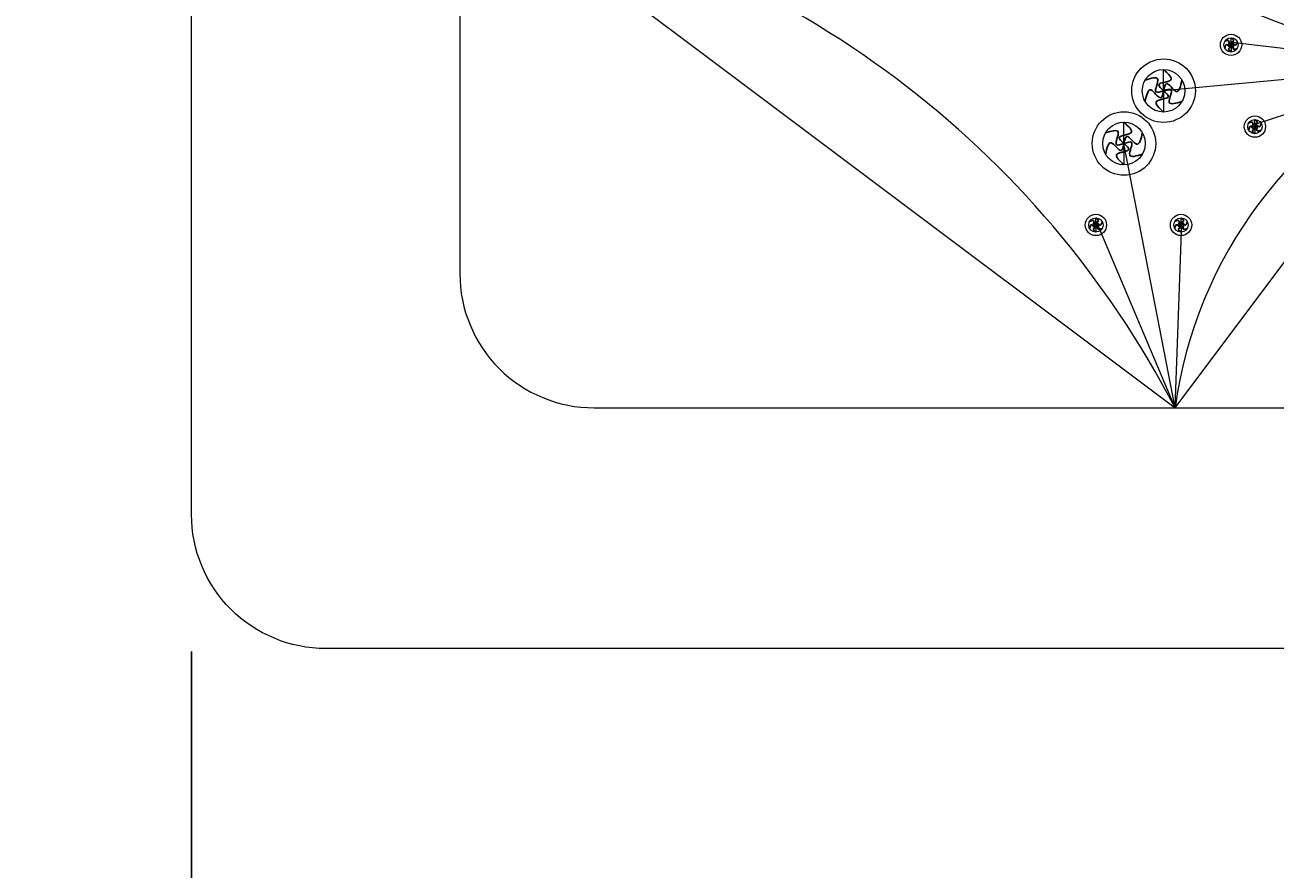
# Model space of a CAD drawing. Units: inches. Extents: x -61 to 1599, y -1316 to 257.
# Tile 99 of 204: x 142 to 170, y -166 to -147. Entities that reach past the tile are written whole.
import ezdxf

# ---------------------------------------------------------------- set-up
doc = ezdxf.new("R2010")
doc.units = ezdxf.units.IN
doc.header["$MEASUREMENT"] = 0
doc.layers.add('A-ANNO-DIMS', color=2, linetype='Continuous', lineweight=18)
doc.layers.add('FURNITURE', color=83, linetype='Continuous', lineweight=18)
doc.layers.add('FUR', color=83, linetype='Continuous')
doc.styles.get("Standard").update_dxf_attribs({"font": 'arial.ttf'})
doc.dimstyles.get("Standard").update_dxf_attribs({"dimtxt": 0.18, "dimasz": 0.18, "dimexe": 0.18, "dimexo": 0.0625, "dimgap": 0.09, "dimtad": 0, "dimtih": 1, "dimtoh": 1, "dimdec": 0, "dimzin": 0, "dimdsep": 46, "dimlunit": 3, "dimtxsty": 'Standard', "dimcen": 0.09, "dimadec": 0, "dimazin": 0, "dimtfac": 1, "dimtdec": 0, "dimtofl": 0, "dimtmove": 0, "dimatfit": 3, "dimfxl": 1, "dimtolj": 1, "dimtzin": 0, "dimarcsym": 0})

# ---------------------------------------------------------------- blocks, each defined once
blk = doc.blocks.new('*U124')
at = {"layer": 'FUR'}
blk.add_open_spline([(0.005, 0.08), (-0.03, 0.048), (-0.098, -0.015), (0.075, -0.018), (0.024, -0.063), (0.005, -0.08)], degree=3, knots=[0, 0, 0, 0, 0.0954578, 0.1898773, 0.2470677, 0.2470677, 0.2470677, 0.2470677], dxfattribs=at)
blk = doc.blocks.new('*U125')
at = {"layer": 'FUR', "transparency": 16777216}
for p, rotation in [((222.173, -79.977), 60), ((222.312, -79.968), 300), ((222.178, -80.056), 120), ((222.25, -80.092), 180), ((222.317, -80.048), 240)]:
    blk.add_blockref('*U124', p, dxfattribs=dict(at, rotation=rotation))
blk.add_blockref('*U124', (222.24, -79.932), dxfattribs=at)
blk = doc.blocks.new('*U134')
at = {"layer": 'FUR'}
blk.add_open_spline([(0.015, 0.238), (-0.088, 0.143), (-0.292, -0.045), (0.224, -0.053), (0.072, -0.187), (0.015, -0.238)], degree=3, knots=[0, 0, 0, 0, 0.2846533, 0.5662105, 0.736751, 0.736751, 0.736751, 0.736751], dxfattribs=at)
blk = doc.blocks.new('*U123')
at = {"layer": 'FUR', "transparency": 16777216}
blk.add_blockref('*U134', (662.716, -238.357), dxfattribs=at)
for p, rotation in [((662.517, -238.489), 60), ((662.929, -238.463), 300), ((662.531, -238.727), 120), ((662.745, -238.833), 180), ((662.944, -238.702), 240)]:
    blk.add_blockref('*U134', p, dxfattribs=dict(at, rotation=rotation))
blk = doc.blocks.new('*U130')
at = {"layer": 'FUR'}
blk.add_open_spline([(0.015, 0.238), (-0.088, 0.143), (-0.292, -0.045), (0.224, -0.053), (0.072, -0.187), (0.015, -0.238)], degree=3, knots=[0, 0, 0, 0, 0.2846533, 0.5662105, 0.736751, 0.736751, 0.736751, 0.736751], dxfattribs=at)
blk = doc.blocks.new('*U131')
at = {"layer": 'FUR', "transparency": 16777216}
blk.add_blockref('*U130', (662.716, -238.357), dxfattribs=at)
for p, rotation in [((662.517, -238.489), 60), ((662.929, -238.463), 300), ((662.531, -238.727), 120), ((662.745, -238.833), 180), ((662.944, -238.702), 240)]:
    blk.add_blockref('*U130', p, dxfattribs=dict(at, rotation=rotation))
blk = doc.blocks.new('*U126')
at = {"layer": 'FUR'}
blk.add_open_spline([(0.005, 0.08), (-0.03, 0.048), (-0.098, -0.015), (0.075, -0.018), (0.024, -0.063), (0.005, -0.08)], degree=3, knots=[0, 0, 0, 0, 0.0954578, 0.1898773, 0.2470677, 0.2470677, 0.2470677, 0.2470677], dxfattribs=at)
blk = doc.blocks.new('*U127')
at = {"layer": 'FUR', "transparency": 16777216}
for p, rotation in [((222.173, -79.977), 60), ((222.312, -79.968), 300), ((222.178, -80.056), 120), ((222.25, -80.092), 180), ((222.317, -80.048), 240)]:
    blk.add_blockref('*U126', p, dxfattribs=dict(at, rotation=rotation))
blk.add_blockref('*U126', (222.24, -79.932), dxfattribs=at)
blk = doc.blocks.new('*U146')
at = {"layer": 'FUR'}
blk.add_open_spline([(0.005, 0.08), (-0.03, 0.048), (-0.098, -0.015), (0.075, -0.018), (0.024, -0.063), (0.005, -0.08)], degree=3, knots=[0, 0, 0, 0, 0.0954578, 0.1898773, 0.2470677, 0.2470677, 0.2470677, 0.2470677], dxfattribs=at)
blk = doc.blocks.new('*U147')
at = {"layer": 'FUR', "transparency": 16777216}
for p, rotation in [((222.173, -79.977), 60), ((222.312, -79.968), 300), ((222.178, -80.056), 120), ((222.25, -80.092), 180), ((222.317, -80.048), 240)]:
    blk.add_blockref('*U146', p, dxfattribs=dict(at, rotation=rotation))
blk.add_blockref('*U146', (222.24, -79.932), dxfattribs=at)
blk = doc.blocks.new('*U144')
at = {"layer": 'FUR'}
blk.add_open_spline([(0.005, 0.08), (-0.03, 0.048), (-0.098, -0.015), (0.075, -0.018), (0.024, -0.063), (0.005, -0.08)], degree=3, knots=[0, 0, 0, 0, 0.0954578, 0.1898773, 0.2470677, 0.2470677, 0.2470677, 0.2470677], dxfattribs=at)
blk = doc.blocks.new('*U145')
at = {"layer": 'FUR', "transparency": 16777216}
for p, rotation in [((222.173, -79.977), 60), ((222.312, -79.968), 300), ((222.178, -80.056), 120), ((222.25, -80.092), 180), ((222.317, -80.048), 240)]:
    blk.add_blockref('*U144', p, dxfattribs=dict(at, rotation=rotation))
blk.add_blockref('*U144', (222.24, -79.932), dxfattribs=at)
blk = doc.blocks.new('SOFA-THREE-SEAT')
for p, q in [((23.243, 13.498), (23.243, 13.658)), ((23.243, 13.498), (23.243, 13.338)), ((27.729, 13.028), (23.263, 13.551)), ((27.729, 13.028), (21.735, 12.472)), ((21.735, 12.472), (21.735, 12.949)), ((27.729, 13.028), (23.795, 11.722)), ((21.735, 12.472), (21.735, 11.996)), ((20.849, 11.292), (20.849, 11.769)), ((23.776, 11.67), (23.776, 11.83)), ((23.776, 11.67), (23.776, 11.51)), ((21.991, 5.382), (20.849, 11.292)), ((20.849, 11.292), (20.849, 10.816)), ((20.221, 9.471), (20.221, 9.631)), ((21.991, 5.382), (20.241, 9.523)), ((21.991, 5.382), (22.145, 9.523)), ((22.125, 9.471), (22.125, 9.631)), ((20.221, 9.471), (20.221, 9.311)), ((22.125, 9.471), (22.125, 9.311))]:
    blk.add_line(p, q)
blk.add_lwpolyline([(78, 8.382), (78, 23, -0.414214), (81, 26), (81, 26, -0.414214), (84, 23), (84, 3, -0.414214), (81, 0), (3, 0, -0.414214), (0, 3), (0, 23, -0.414214), (3, 26), (3, 26, -0.414214), (6, 23), (6, 8.382, 0.414214), (9, 5.382), (75, 5.382, 0.414214)], format="xyb", close=True)
blk.add_lwpolyline([(27.729, 13.028), (12.664, 24.333), (6.926, 16.687), (21.991, 5.382)], close=True)
for centre, radius in [((23.243, 13.498), 0.238), ((23.243, 13.498), 0.16), ((21.735, 12.472), 0.71), ((21.735, 12.472), 0.476), ((20.849, 11.292), 0.71), ((20.849, 11.292), 0.476), ((23.776, 11.67), 0.238), ((23.776, 11.67), 0.16), ((20.221, 9.471), 0.238), ((20.221, 9.471), 0.16), ((22.125, 9.471), 0.238), ((22.125, 9.471), 0.16)]:
    blk.add_circle(centre, radius)
for centre, radius, start, end in [((31.951, 34.345), 21.731, 207.4316, 258.7956), ((2.703, -4.63), 21.731, 27.4316, 78.7956), ((31.717, 4.059), 9.816, 113.9742, 172.253)]:
    blk.add_arc(centre, radius, start, end)
at = {"xscale": -1, "rotation": 180}
for name, p in [('*U147', (-199.001, -66.514)), ('*U131', (-640.996, -226.123)), ('*U123', (-641.881, -227.303)), ('*U145', (-198.469, -68.342)), ('*U125', (-202.024, -70.541)), ('*U127', (-200.12, -70.541))]:
    blk.add_blockref(name, p, dxfattribs=at)
blk = doc.blocks.new('*D670')
at = {"layer": 'A-ANNO-DIMS', "color": 0, "lineweight": -2, "transparency": 16777216}
for p, q in [((145.375, -161.442), (145.375, -174.159)), ((229.375, -161.442), (229.375, -174.159)), ((145.555, -173.979), (186.47, -173.979)), ((229.195, -173.979), (188.279, -173.979))]:
    blk.add_line(p, q, dxfattribs=at)
at = {"layer": 'A-ANNO-DIMS', "color": 0, "transparency": 16777216}
for points in [[(145.555, -173.949), (145.555, -174.009), (145.375, -173.979)], [(229.195, -173.949), (229.195, -174.009), (229.375, -173.979)]]:
    blk.add_solid(points, dxfattribs=at)
at = {"layer": 'DEFPOINTS', "color": 0, "transparency": 16777216}
for p in [(145.375, -161.379), (229.375, -161.379), (229.375, -173.979)]:
    blk.add_point(p, dxfattribs=at)
at = {"layer": 'A-ANNO-DIMS', "color": 0, "transparency": 16777216, "insert": (187.375, -173.979), "char_height": 0.18, "attachment_point": 5}
blk.add_mtext('\\A1;SOFA 84 TYP.', dxfattribs=at)
blk = doc.blocks.new('*D687')
at = {"layer": 'A-ANNO-DIMS', "color": 0, "lineweight": -2, "transparency": 16777216}
for p, q in [((289.418, 181.677), (-61.077, 181.677)), ((-60.897, 181.497), (-60.897, -528.952)), ((-60.897, -1239.765), (-60.897, -529.316)), ((319.64, -1239.945), (-61.077, -1239.945))]:
    blk.add_line(p, q, dxfattribs=at)
at = {"layer": 'A-ANNO-DIMS', "color": 0, "transparency": 16777216}
for points in [[(-60.927, 181.497), (-60.867, 181.497), (-60.897, 181.677)], [(-60.927, -1239.765), (-60.867, -1239.765), (-60.897, -1239.945)]]:
    blk.add_solid(points, dxfattribs=at)
at = {"layer": 'DEFPOINTS', "color": 0, "transparency": 16777216}
for p in [(289.481, 181.677), (-60.897, -1239.945), (319.703, -1239.945)]:
    blk.add_point(p, dxfattribs=at)
at = {"layer": 'A-ANNO-DIMS', "color": 0, "transparency": 16777216, "insert": (-60.897, -529.134), "char_height": 0.18, "attachment_point": 5}
blk.add_mtext('\\A1;1421.6', dxfattribs=at)
blk = doc.blocks.new('*D700')
at = {"layer": 'A-ANNO-DIMS', "color": 0, "lineweight": -2, "transparency": 16777216}
for p, q in [((14.703, -616.882), (14.703, 257.457)), ((179.752, -616.882), (179.752, 257.457)), ((14.883, 257.277), (96.772, 257.277)), ((179.572, 257.277), (97.683, 257.277))]:
    blk.add_line(p, q, dxfattribs=at)
at = {"layer": 'A-ANNO-DIMS', "color": 0, "transparency": 16777216}
for points in [[(14.883, 257.307), (14.883, 257.247), (14.703, 257.277)], [(179.572, 257.307), (179.572, 257.247), (179.752, 257.277)]]:
    blk.add_solid(points, dxfattribs=at)
at = {"layer": 'DEFPOINTS', "color": 0, "transparency": 16777216}
for p in [(179.752, 257.277), (14.703, -616.945), (179.752, -616.945)]:
    blk.add_point(p, dxfattribs=at)
at = {"layer": 'A-ANNO-DIMS', "color": 0, "transparency": 16777216, "insert": (97.227, 257.277), "char_height": 0.18, "attachment_point": 5}
blk.add_mtext('\\A1;165.05', dxfattribs=at)

msp = doc.modelspace()

# ---------------------------------------------------------------- block references
at = {"layer": 'FURNITURE'}
msp.add_blockref('SOFA-THREE-SEAT', (145.375, -161.379), dxfattribs=at)

# ---------------------------------------------------------------- dimensions: what is measured, and where the dimension line sits
at = {"layer": 'A-ANNO-DIMS'}
dim = msp.add_linear_dim(base=(179.7521, 257.2771), p1=(14.7028, -616.9446), p2=(179.7521, -616.9446), dimstyle='Standard', override={"dimdec": 2, "dimlfac": 1, "dimrnd": 0, "dimzin": 0, "dimdsep": 46, "dimlunit": 2}, dxfattribs=at)
dim.commit()
dim.dimension.update_dxf_attribs({"geometry": '*D700', "text_midpoint": (97.2274, 257.2771)})
dim = msp.add_linear_dim(base=(-60.8972, -1239.9446), p1=(289.4807, 181.6771), p2=(319.7028, -1239.9446), angle=90, dimstyle='Standard', override={"dimdec": 1, "dimlfac": 1, "dimrnd": 0, "dimzin": 0, "dimdsep": 46, "dimlunit": 2}, dxfattribs=at)
dim.commit()
dim.dimension.update_dxf_attribs({"geometry": '*D687', "text_midpoint": (-60.8972, -529.1337)})
dim = msp.add_linear_dim(base=(229.3746, -173.9792), p1=(145.3746, -161.3792), p2=(229.3746, -161.3792), text='SOFA <> TYP.', dimstyle='Standard', override={"dimdec": 0, "dimlfac": 1, "dimrnd": 0, "dimzin": 0, "dimdsep": 46, "dimlunit": 2}, dxfattribs=at)
dim.commit()
dim.dimension.update_dxf_attribs({"geometry": '*D670', "text_midpoint": (187.3746, -173.9792)})

doc.saveas('drawing.dxf')
